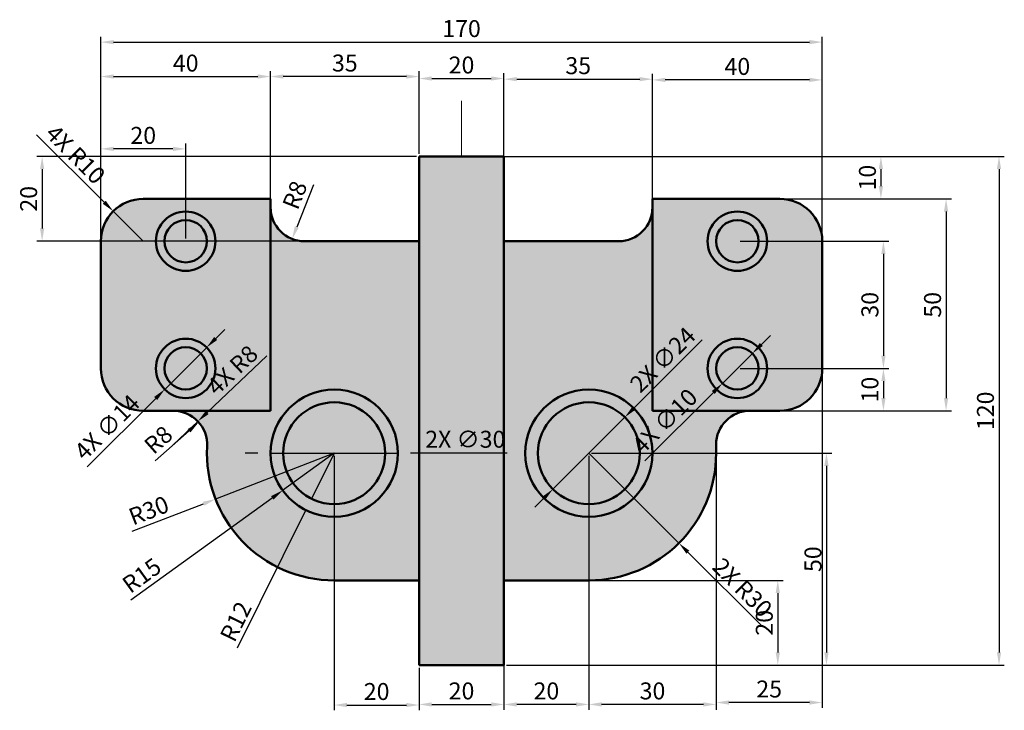
# Model space of a CAD drawing. Units: millimetres. Extents: x 624 to 856, y 718 to 881.
import ezdxf

# ---------------------------------------------------------------- set-up
doc = ezdxf.new("R2010")
doc.units = ezdxf.units.MM
doc.linetypes.add('CENTER', pattern=[50.8, 31.75, -6.35, 6.35, -6.35])
for name, color, linetype, lineweight in [('M-CNTR', 4, 'CENTER', 18), ('M-DIMS', 2, 'Continuous', 25), ('M-HATC', 8, 'Continuous', 18), ('M-OUTL', 7, 'Continuous', 50)]:
    doc.layers.add(name, color=color, linetype=linetype, lineweight=lineweight)
doc.styles.get("Standard").update_dxf_attribs({"font": 'arial.ttf'})
doc.dimstyles.new('ISO-25', dxfattribs={"dimtxt": 4, "dimasz": 3, "dimexe": 1.25, "dimexo": 0.625, "dimtad": 1, "dimdec": 1, "dimtxsty": 'Standard', "dimcen": 2.5, "dimadec": 0, "dimazin": 0, "dimtfac": 1, "dimtdec": 1, "dimtmove": 0, "dimatfit": 3, "dimfxl": 1, "dimarcsym": 0})

# ---------------------------------------------------------------- blocks, each defined once
blk = doc.blocks.new('*D1')
at = {"layer": 'Defpoints', "color": 0, "transparency": 16777216}
for p in [(698.17, 778.8), (718.17, 728.8), (718.17, 719.4)]:
    blk.add_point(p, dxfattribs=at)
at = {"layer": 'M-DIMS', "color": 0, "lineweight": -2, "transparency": 16777216}
for p, q in [((698.17, 778.17), (698.17, 718.15)), ((718.17, 728.17), (718.17, 718.15)), ((701.17, 719.4), (715.17, 719.4))]:
    blk.add_line(p, q, dxfattribs=at)
at = {"layer": 'M-DIMS', "color": 0, "transparency": 16777216}
for points in [[(701.17, 719.9), (701.17, 718.9), (698.17, 719.4)], [(715.17, 719.9), (715.17, 718.9), (718.17, 719.4)]]:
    blk.add_solid(points, dxfattribs=at)
at = {"layer": 'M-DIMS', "color": 0, "transparency": 16777216, "insert": (708.17, 722.07), "char_height": 4, "attachment_point": 5}
blk.add_mtext('20', dxfattribs=at)
blk = doc.blocks.new('*D2')
at = {"layer": 'Defpoints', "color": 0, "transparency": 16777216}
for p in [(738.17, 728.8), (718.17, 723.16), (738.17, 719.54)]:
    blk.add_point(p, dxfattribs=at)
at = {"layer": 'M-DIMS', "color": 0, "lineweight": -2, "transparency": 16777216}
for p, q in [((738.17, 728.17), (738.17, 718.29)), ((718.17, 722.54), (718.17, 718.29)), ((721.17, 719.54), (735.17, 719.54))]:
    blk.add_line(p, q, dxfattribs=at)
at = {"layer": 'M-DIMS', "color": 0, "transparency": 16777216}
for points in [[(721.17, 720.04), (721.17, 719.04), (718.17, 719.54)], [(735.17, 720.04), (735.17, 719.04), (738.17, 719.54)]]:
    blk.add_solid(points, dxfattribs=at)
at = {"layer": 'M-DIMS', "color": 0, "transparency": 16777216, "insert": (728.17, 722.21), "char_height": 4, "attachment_point": 5}
blk.add_mtext('20', dxfattribs=at)
blk = doc.blocks.new('*D3')
at = {"layer": 'Defpoints', "color": 0, "transparency": 16777216}
for p in [(758.17, 778.8), (738.17, 732.79), (738.17, 719.54)]:
    blk.add_point(p, dxfattribs=at)
at = {"layer": 'M-DIMS', "color": 0, "lineweight": -2, "transparency": 16777216}
for p, q in [((758.17, 778.17), (758.17, 718.29)), ((738.17, 732.16), (738.17, 718.29)), ((755.17, 719.54), (741.17, 719.54))]:
    blk.add_line(p, q, dxfattribs=at)
at = {"layer": 'M-DIMS', "color": 0, "transparency": 16777216}
for points in [[(741.17, 720.04), (741.17, 719.04), (738.17, 719.54)], [(755.17, 720.04), (755.17, 719.04), (758.17, 719.54)]]:
    blk.add_solid(points, dxfattribs=at)
at = {"layer": 'M-DIMS', "color": 0, "transparency": 16777216, "insert": (748.17, 722.21), "char_height": 4, "attachment_point": 5}
blk.add_mtext('20', dxfattribs=at)
blk = doc.blocks.new('*D4')
at = {"layer": 'Defpoints', "color": 0, "transparency": 16777216}
for p in [(788.17, 778.8), (758.17, 736.06), (758.17, 719.54)]:
    blk.add_point(p, dxfattribs=at)
at = {"layer": 'M-DIMS', "color": 0, "lineweight": -2, "transparency": 16777216}
for p, q in [((788.17, 778.17), (788.17, 718.29)), ((758.17, 735.44), (758.17, 718.29)), ((785.17, 719.54), (761.17, 719.54))]:
    blk.add_line(p, q, dxfattribs=at)
at = {"layer": 'M-DIMS', "color": 0, "transparency": 16777216}
for points in [[(761.17, 720.04), (761.17, 719.04), (758.17, 719.54)], [(785.17, 720.04), (785.17, 719.04), (788.17, 719.54)]]:
    blk.add_solid(points, dxfattribs=at)
at = {"layer": 'M-DIMS', "color": 0, "transparency": 16777216, "insert": (773.17, 722.21), "char_height": 4, "attachment_point": 5}
blk.add_mtext('30', dxfattribs=at)
blk = doc.blocks.new('*D5')
at = {"layer": 'Defpoints', "color": 0, "transparency": 16777216}
for p in [(758.17, 778.8), (738.17, 728.8), (814.17, 728.8)]:
    blk.add_point(p, dxfattribs=at)
at = {"layer": 'M-DIMS', "color": 0, "lineweight": -2, "transparency": 16777216}
for p, q in [((758.8, 778.8), (815.42, 778.8)), ((814.17, 775.8), (814.17, 731.8)), ((738.8, 728.8), (815.42, 728.8))]:
    blk.add_line(p, q, dxfattribs=at)
at = {"layer": 'M-DIMS', "color": 0, "transparency": 16777216}
for points in [[(813.67, 775.8), (814.67, 775.8), (814.17, 778.8)], [(813.67, 731.8), (814.67, 731.8), (814.17, 728.8)]]:
    blk.add_solid(points, dxfattribs=at)
at = {"layer": 'M-DIMS', "color": 0, "transparency": 16777216, "insert": (811.51, 753.8), "char_height": 4, "attachment_point": 5, "rotation": 90}
blk.add_mtext('50', dxfattribs=at)
blk = doc.blocks.new('*D6')
at = {"layer": 'Defpoints', "color": 0, "transparency": 16777216}
for p in [(749.94, 748.8), (749.94, 728.8), (802.7, 728.8)]:
    blk.add_point(p, dxfattribs=at)
at = {"layer": 'M-DIMS', "color": 0, "lineweight": -2, "transparency": 16777216}
for p, q in [((750.56, 748.8), (803.95, 748.8)), ((802.7, 745.8), (802.7, 731.8)), ((750.56, 728.8), (803.95, 728.8))]:
    blk.add_line(p, q, dxfattribs=at)
at = {"layer": 'M-DIMS', "color": 0, "transparency": 16777216}
for points in [[(802.2, 745.8), (803.2, 745.8), (802.7, 748.8)], [(802.2, 731.8), (803.2, 731.8), (802.7, 728.8)]]:
    blk.add_solid(points, dxfattribs=at)
at = {"layer": 'M-DIMS', "color": 0, "transparency": 16777216, "insert": (800.04, 738.8), "char_height": 4, "attachment_point": 5, "rotation": 90}
blk.add_mtext('20', dxfattribs=at)
blk = doc.blocks.new('*D7')
at = {"layer": 'Defpoints', "color": 0, "transparency": 16777216}
for p in [(793.17, 798.8), (800.11, 788.8), (827.59, 788.8)]:
    blk.add_point(p, dxfattribs=at)
at = {"layer": 'M-DIMS', "color": 0, "lineweight": -2, "transparency": 16777216}
for p, q in [((793.8, 798.8), (828.84, 798.8)), ((827.59, 795.8), (827.59, 791.8)), ((800.74, 788.8), (828.84, 788.8))]:
    blk.add_line(p, q, dxfattribs=at)
at = {"layer": 'M-DIMS', "color": 0, "transparency": 16777216}
for points in [[(827.09, 795.8), (828.09, 795.8), (827.59, 798.8)], [(827.09, 791.8), (828.09, 791.8), (827.59, 788.8)]]:
    blk.add_solid(points, dxfattribs=at)
at = {"layer": 'M-DIMS', "color": 0, "transparency": 16777216, "insert": (824.92, 793.8), "char_height": 4, "attachment_point": 5, "rotation": 90}
blk.add_mtext('10', dxfattribs=at)
blk = doc.blocks.new('*D8')
at = {"layer": 'Defpoints', "color": 0, "transparency": 16777216}
for p in [(793.17, 828.8), (793.17, 798.8), (827.59, 798.8)]:
    blk.add_point(p, dxfattribs=at)
at = {"layer": 'M-DIMS', "color": 0, "lineweight": -2, "transparency": 16777216}
for p, q in [((793.8, 828.8), (828.84, 828.8)), ((827.59, 825.8), (827.59, 801.8)), ((793.8, 798.8), (828.84, 798.8))]:
    blk.add_line(p, q, dxfattribs=at)
at = {"layer": 'M-DIMS', "color": 0, "transparency": 16777216}
for points in [[(827.09, 825.8), (828.09, 825.8), (827.59, 828.8)], [(827.09, 801.8), (828.09, 801.8), (827.59, 798.8)]]:
    blk.add_solid(points, dxfattribs=at)
at = {"layer": 'M-DIMS', "color": 0, "transparency": 16777216, "insert": (824.92, 813.8), "char_height": 4, "attachment_point": 5, "rotation": 90}
blk.add_mtext('30', dxfattribs=at)
blk = doc.blocks.new('*D9')
at = {"layer": 'Defpoints', "color": 0, "transparency": 16777216}
for p in [(794.11, 838.8), (798.04, 788.8), (842.36, 788.8)]:
    blk.add_point(p, dxfattribs=at)
at = {"layer": 'M-DIMS', "color": 0, "lineweight": -2, "transparency": 16777216}
for p, q in [((794.74, 838.8), (843.61, 838.8)), ((842.36, 835.8), (842.36, 791.8)), ((798.66, 788.8), (843.61, 788.8))]:
    blk.add_line(p, q, dxfattribs=at)
at = {"layer": 'M-DIMS', "color": 0, "transparency": 16777216}
for points in [[(841.86, 835.8), (842.86, 835.8), (842.36, 838.8)], [(841.86, 791.8), (842.86, 791.8), (842.36, 788.8)]]:
    blk.add_solid(points, dxfattribs=at)
at = {"layer": 'M-DIMS', "color": 0, "transparency": 16777216, "insert": (839.69, 813.8), "char_height": 4, "attachment_point": 5, "rotation": 90}
blk.add_mtext('50', dxfattribs=at)
blk = doc.blocks.new('*D10')
at = {"layer": 'Defpoints', "color": 0, "transparency": 16777216}
for p in [(728.17, 848.8), (795.5, 728.8), (854.83, 728.8)]:
    blk.add_point(p, dxfattribs=at)
at = {"layer": 'M-DIMS', "color": 0, "lineweight": -2, "transparency": 16777216}
for p, q in [((728.8, 848.8), (856.08, 848.8)), ((854.83, 845.8), (854.83, 731.8)), ((796.12, 728.8), (856.08, 728.8))]:
    blk.add_line(p, q, dxfattribs=at)
at = {"layer": 'M-DIMS', "color": 0, "transparency": 16777216}
for points in [[(854.33, 845.8), (855.33, 845.8), (854.83, 848.8)], [(854.33, 731.8), (855.33, 731.8), (854.83, 728.8)]]:
    blk.add_solid(points, dxfattribs=at)
at = {"layer": 'M-DIMS', "color": 0, "transparency": 16777216, "insert": (852.16, 788.8), "char_height": 4, "attachment_point": 5, "rotation": 90}
blk.add_mtext('120', dxfattribs=at)
blk = doc.blocks.new('*D11')
at = {"layer": 'Defpoints', "color": 0, "transparency": 16777216}
for p in [(683.17, 867.64), (643.17, 820.21), (683.17, 818.82)]:
    blk.add_point(p, dxfattribs=at)
at = {"layer": 'M-DIMS', "color": 0, "lineweight": -2, "transparency": 16777216}
for p, q in [((643.17, 820.83), (643.17, 868.89)), ((683.17, 819.44), (683.17, 868.89)), ((646.17, 867.64), (680.17, 867.64))]:
    blk.add_line(p, q, dxfattribs=at)
at = {"layer": 'M-DIMS', "color": 0, "transparency": 16777216}
for points in [[(646.17, 868.14), (646.17, 867.14), (643.17, 867.64)], [(680.17, 868.14), (680.17, 867.14), (683.17, 867.64)]]:
    blk.add_solid(points, dxfattribs=at)
at = {"layer": 'M-DIMS', "color": 0, "transparency": 16777216, "insert": (663.17, 870.3), "char_height": 4, "attachment_point": 5}
blk.add_mtext('40', dxfattribs=at)
blk = doc.blocks.new('*D12')
at = {"layer": 'Defpoints', "color": 0, "transparency": 16777216}
for p in [(683.17, 867.64), (683.17, 848.8), (718.17, 848.8)]:
    blk.add_point(p, dxfattribs=at)
at = {"layer": 'M-DIMS', "color": 0, "lineweight": -2, "transparency": 16777216}
for p, q in [((683.17, 849.42), (683.17, 868.89)), ((718.17, 849.42), (718.17, 868.89)), ((715.17, 867.64), (686.17, 867.64))]:
    blk.add_line(p, q, dxfattribs=at)
at = {"layer": 'M-DIMS', "color": 0, "transparency": 16777216}
for points in [[(686.17, 868.14), (686.17, 867.14), (683.17, 867.64)], [(715.17, 868.14), (715.17, 867.14), (718.17, 867.64)]]:
    blk.add_solid(points, dxfattribs=at)
at = {"layer": 'M-DIMS', "color": 0, "transparency": 16777216, "insert": (700.67, 870.31), "char_height": 4, "attachment_point": 5}
blk.add_mtext('35', dxfattribs=at)
blk = doc.blocks.new('*D13')
at = {"layer": 'Defpoints', "color": 0, "transparency": 16777216}
for p in [(738.17, 867.17), (718.17, 848.8), (738.17, 848.8)]:
    blk.add_point(p, dxfattribs=at)
at = {"layer": 'M-DIMS', "color": 0, "lineweight": -2, "transparency": 16777216}
for p, q in [((718.17, 849.42), (718.17, 868.42)), ((738.17, 849.42), (738.17, 868.42)), ((721.17, 867.17), (735.17, 867.17))]:
    blk.add_line(p, q, dxfattribs=at)
at = {"layer": 'M-DIMS', "color": 0, "transparency": 16777216}
for points in [[(721.17, 867.67), (721.17, 866.67), (718.17, 867.17)], [(735.17, 867.67), (735.17, 866.67), (738.17, 867.17)]]:
    blk.add_solid(points, dxfattribs=at)
at = {"layer": 'M-DIMS', "color": 0, "transparency": 16777216, "insert": (728.17, 869.84), "char_height": 4, "attachment_point": 5}
blk.add_mtext('20', dxfattribs=at)
blk = doc.blocks.new('*D14')
at = {"layer": 'Defpoints', "color": 0, "transparency": 16777216}
for p in [(773.17, 867.02), (738.17, 839.17), (773.17, 838.8)]:
    blk.add_point(p, dxfattribs=at)
at = {"layer": 'M-DIMS', "color": 0, "lineweight": -2, "transparency": 16777216}
for p, q in [((738.17, 839.79), (738.17, 868.27)), ((773.17, 839.42), (773.17, 868.27)), ((741.17, 867.02), (770.17, 867.02))]:
    blk.add_line(p, q, dxfattribs=at)
at = {"layer": 'M-DIMS', "color": 0, "transparency": 16777216}
for points in [[(741.17, 867.52), (741.17, 866.52), (738.17, 867.02)], [(770.17, 867.52), (770.17, 866.52), (773.17, 867.02)]]:
    blk.add_solid(points, dxfattribs=at)
at = {"layer": 'M-DIMS', "color": 0, "transparency": 16777216, "insert": (755.67, 869.69), "char_height": 4, "attachment_point": 5}
blk.add_mtext('35', dxfattribs=at)
blk = doc.blocks.new('*D15')
at = {"layer": 'Defpoints', "color": 0, "transparency": 16777216}
for p in [(773.17, 866.84), (773.17, 818.33), (813.17, 818.33)]:
    blk.add_point(p, dxfattribs=at)
at = {"layer": 'M-DIMS', "color": 0, "lineweight": -2, "transparency": 16777216}
for p, q in [((773.17, 818.95), (773.17, 868.09)), ((813.17, 818.95), (813.17, 868.09)), ((810.17, 866.84), (776.17, 866.84))]:
    blk.add_line(p, q, dxfattribs=at)
at = {"layer": 'M-DIMS', "color": 0, "transparency": 16777216}
for points in [[(776.17, 867.34), (776.17, 866.34), (773.17, 866.84)], [(810.17, 867.34), (810.17, 866.34), (813.17, 866.84)]]:
    blk.add_solid(points, dxfattribs=at)
at = {"layer": 'M-DIMS', "color": 0, "transparency": 16777216, "insert": (793.17, 869.51), "char_height": 4, "attachment_point": 5}
blk.add_mtext('40', dxfattribs=at)
blk = doc.blocks.new('*D16')
at = {"layer": 'Defpoints', "color": 0, "transparency": 16777216}
for p in [(643.17, 850.58), (663.17, 828.8), (643.17, 816.04)]:
    blk.add_point(p, dxfattribs=at)
at = {"layer": 'M-DIMS', "color": 0, "lineweight": -2, "transparency": 16777216}
for p, q in [((643.17, 816.67), (643.17, 851.83)), ((663.17, 829.42), (663.17, 851.83)), ((660.17, 850.58), (646.17, 850.58))]:
    blk.add_line(p, q, dxfattribs=at)
at = {"layer": 'M-DIMS', "color": 0, "transparency": 16777216}
for points in [[(646.17, 851.08), (646.17, 850.08), (643.17, 850.58)], [(660.17, 851.08), (660.17, 850.08), (663.17, 850.58)]]:
    blk.add_solid(points, dxfattribs=at)
at = {"layer": 'M-DIMS', "color": 0, "transparency": 16777216, "insert": (653.17, 853.24), "char_height": 4, "attachment_point": 5}
blk.add_mtext('20', dxfattribs=at)
blk = doc.blocks.new('*D17')
at = {"layer": 'Defpoints', "color": 0, "transparency": 16777216}
for p in [(691.17, 836.8), (688.24, 829.35)]:
    blk.add_point(p, dxfattribs=at)
at = {"layer": 'M-DIMS', "color": 0, "lineweight": -2, "transparency": 16777216}
blk.add_line((693.27, 842.11), (689.34, 832.14), dxfattribs=at)
at = {"layer": 'M-DIMS', "color": 0, "transparency": 16777216}
blk.add_solid([(688.88, 832.33), (689.81, 831.96), (688.24, 829.35)], dxfattribs=at)
at = {"layer": 'M-DIMS', "color": 0, "transparency": 16777216, "insert": (689.37, 839.5), "char_height": 4, "attachment_point": 5, "rotation": 68.4911}
blk.add_mtext('R8', dxfattribs=at)
blk = doc.blocks.new('*D18')
at = {"layer": 'Defpoints', "color": 0, "transparency": 16777216}
for p in [(698.17, 778.8), (686.01, 770.02)]:
    blk.add_point(p, dxfattribs=at)
at = {"layer": 'M-DIMS', "color": 0, "lineweight": -2, "transparency": 16777216}
for p, q in [((698.17, 778.8), (686.01, 770.02)), ((650.28, 744.22), (683.58, 768.26))]:
    blk.add_line(p, q, dxfattribs=at)
at = {"layer": 'M-DIMS', "color": 0, "transparency": 16777216}
blk.add_solid([(683.29, 768.67), (683.87, 767.85), (686.01, 770.02)], dxfattribs=at)
at = {"layer": 'M-DIMS', "color": 0, "transparency": 16777216, "insert": (653.11, 749.55), "char_height": 4, "attachment_point": 5, "rotation": 35.8278}
blk.add_mtext('R15', dxfattribs=at)
blk = doc.blocks.new('*D19')
at = {"layer": 'Defpoints', "color": 0, "transparency": 16777216}
for p in [(698.17, 778.8), (692.85, 768.04)]:
    blk.add_point(p, dxfattribs=at)
at = {"layer": 'M-DIMS', "color": 0, "lineweight": -2, "transparency": 16777216}
for p, q in [((698.17, 778.8), (692.85, 768.04)), ((675.41, 732.87), (691.51, 765.36))]:
    blk.add_line(p, q, dxfattribs=at)
at = {"layer": 'M-DIMS', "color": 0, "transparency": 16777216}
blk.add_solid([(691.06, 765.58), (691.96, 765.13), (692.85, 768.04)], dxfattribs=at)
at = {"layer": 'M-DIMS', "color": 0, "transparency": 16777216, "insert": (675.44, 738.87), "char_height": 4, "attachment_point": 5, "rotation": 63.6308}
blk.add_mtext('R12', dxfattribs=at)
blk = doc.blocks.new('*D20')
at = {"layer": 'Defpoints', "color": 0, "transparency": 16777216}
for p in [(698.17, 778.8), (670.2, 767.97)]:
    blk.add_point(p, dxfattribs=at)
at = {"layer": 'M-DIMS', "color": 0, "lineweight": -2, "transparency": 16777216}
for p, q in [((698.17, 778.8), (670.2, 767.97)), ((650.58, 760.38), (667.4, 766.89))]:
    blk.add_line(p, q, dxfattribs=at)
at = {"layer": 'M-DIMS', "color": 0, "transparency": 16777216}
blk.add_solid([(667.22, 767.35), (667.58, 766.42), (670.2, 767.97)], dxfattribs=at)
at = {"layer": 'M-DIMS', "color": 0, "transparency": 16777216, "insert": (654.65, 764.81), "char_height": 4, "attachment_point": 5, "rotation": 21.1564}
blk.add_mtext('R30', dxfattribs=at)
blk = doc.blocks.new('*D21')
at = {"layer": 'Defpoints', "color": 0, "transparency": 16777216}
for p in [(666.22, 786.09), (660.23, 780.8)]:
    blk.add_point(p, dxfattribs=at)
at = {"layer": 'M-DIMS', "color": 0, "lineweight": -2, "transparency": 16777216}
blk.add_line((655.95, 777.02), (663.98, 784.11), dxfattribs=at)
at = {"layer": 'M-DIMS', "color": 0, "transparency": 16777216}
blk.add_solid([(663.64, 784.48), (664.31, 783.73), (666.22, 786.09)], dxfattribs=at)
at = {"layer": 'M-DIMS', "color": 0, "transparency": 16777216, "insert": (657.07, 781.57), "char_height": 4, "attachment_point": 5, "rotation": 41.4423}
blk.add_mtext('R8', dxfattribs=at)
blk = doc.blocks.new('*D22')
at = {"layer": 'Defpoints', "color": 0, "transparency": 16777216}
for p in [(813.17, 813.8), (788.17, 723.81), (788.17, 719.99)]:
    blk.add_point(p, dxfattribs=at)
at = {"layer": 'M-DIMS', "color": 0, "lineweight": -2, "transparency": 16777216}
for p, q in [((813.17, 813.17), (813.17, 718.74)), ((788.17, 723.19), (788.17, 718.74)), ((810.17, 719.99), (791.17, 719.99))]:
    blk.add_line(p, q, dxfattribs=at)
at = {"layer": 'M-DIMS', "color": 0, "transparency": 16777216}
for points in [[(791.17, 720.49), (791.17, 719.49), (788.17, 719.99)], [(810.17, 720.49), (810.17, 719.49), (813.17, 719.99)]]:
    blk.add_solid(points, dxfattribs=at)
at = {"layer": 'M-DIMS', "color": 0, "transparency": 16777216, "insert": (800.67, 722.66), "char_height": 4, "attachment_point": 5}
blk.add_mtext('25', dxfattribs=at)
blk = doc.blocks.new('CLEVIS-LUG-40X50-2HOLE')
for p, q in [((10, 50), (40, 50)), ((40, 0), (40, 50)), ((0, 40), (0, 10)), ((10, 0), (40, 0))]:
    blk.add_line(p, q)
for centre, radius in [((20, 40), 7), ((20, 40), 5), ((20, 10), 7), ((20, 10), 5)]:
    blk.add_circle(centre, radius)
for centre, start, end in [((10, 40), 90, 180), ((10, 10), 180, 270)]:
    blk.add_arc(centre, 10, start, end)
blk = doc.blocks.new('PLATE-BORE-D24-D30')
for radius in [15, 12]:
    blk.add_circle((15, 15), radius)
blk = doc.blocks.new('*D25')
at = {"layer": 'Defpoints', "color": 0, "transparency": 16777216}
for p in [(813.17, 875.76), (643.17, 828.8), (813.17, 828.8)]:
    blk.add_point(p, dxfattribs=at)
at = {"layer": 'M-DIMS', "color": 0, "lineweight": -2, "transparency": 16777216}
for p, q in [((643.17, 829.42), (643.17, 877.01)), ((646.17, 875.76), (810.17, 875.76)), ((813.17, 829.42), (813.17, 877.01))]:
    blk.add_line(p, q, dxfattribs=at)
at = {"layer": 'M-DIMS', "color": 0, "transparency": 16777216}
for points in [[(646.17, 876.26), (646.17, 875.26), (643.17, 875.76)], [(810.17, 876.26), (810.17, 875.26), (813.17, 875.76)]]:
    blk.add_solid(points, dxfattribs=at)
at = {"layer": 'M-DIMS', "color": 0, "transparency": 16777216, "insert": (728.17, 878.43), "char_height": 4, "attachment_point": 5}
blk.add_mtext('170', dxfattribs=at)
blk = doc.blocks.new('*D26')
at = {"layer": 'Defpoints', "color": 0, "transparency": 16777216}
for p in [(738.17, 848.8), (803.17, 838.8), (827, 838.8)]:
    blk.add_point(p, dxfattribs=at)
at = {"layer": 'M-DIMS', "color": 0, "lineweight": -2, "transparency": 16777216}
for p, q in [((738.8, 848.8), (828.25, 848.8)), ((827, 845.8), (827, 841.8)), ((803.8, 838.8), (828.25, 838.8))]:
    blk.add_line(p, q, dxfattribs=at)
at = {"layer": 'M-DIMS', "color": 0, "transparency": 16777216}
for points in [[(826.5, 845.8), (827.5, 845.8), (827, 848.8)], [(826.5, 841.8), (827.5, 841.8), (827, 838.8)]]:
    blk.add_solid(points, dxfattribs=at)
at = {"layer": 'M-DIMS', "color": 0, "transparency": 16777216, "insert": (824.34, 843.8), "char_height": 4, "attachment_point": 5, "rotation": 90}
blk.add_mtext('10', dxfattribs=at)
blk = doc.blocks.new('*D27')
at = {"layer": 'Defpoints', "color": 0, "transparency": 16777216}
for p in [(718.17, 848.8), (629.34, 828.8), (718.17, 828.8)]:
    blk.add_point(p, dxfattribs=at)
at = {"layer": 'M-DIMS', "color": 0, "lineweight": -2, "transparency": 16777216}
for p, q in [((717.55, 848.8), (628.09, 848.8)), ((629.34, 845.8), (629.34, 831.8)), ((717.55, 828.8), (628.09, 828.8))]:
    blk.add_line(p, q, dxfattribs=at)
at = {"layer": 'M-DIMS', "color": 0, "transparency": 16777216}
for points in [[(628.84, 845.8), (629.84, 845.8), (629.34, 848.8)], [(628.84, 831.8), (629.84, 831.8), (629.34, 828.8)]]:
    blk.add_solid(points, dxfattribs=at)
at = {"layer": 'M-DIMS', "color": 0, "transparency": 16777216, "insert": (626.68, 838.8), "char_height": 4, "attachment_point": 5, "rotation": 90}
blk.add_mtext('20', dxfattribs=at)
blk = doc.blocks.new('*D28')
at = {"layer": 'Defpoints', "color": 0, "transparency": 16777216}
for p in [(758.17, 778.8), (779.39, 757.58)]:
    blk.add_point(p, dxfattribs=at)
at = {"layer": 'M-DIMS', "color": 0, "lineweight": -2, "transparency": 16777216}
for p, q in [((758.17, 778.8), (779.39, 757.58)), ((799, 737.98), (781.51, 755.46))]:
    blk.add_line(p, q, dxfattribs=at)
at = {"layer": 'M-DIMS', "color": 0, "transparency": 16777216}
blk.add_solid([(781.86, 755.82), (781.16, 755.11), (779.39, 757.58)], dxfattribs=at)
at = {"layer": 'M-DIMS', "color": 0, "transparency": 16777216, "insert": (794, 746.74), "char_height": 4, "attachment_point": 5, "rotation": 314.9999}
blk.add_mtext('2X R30', dxfattribs=at)
blk = doc.blocks.new('*D29')
at = {"layer": 'Defpoints', "color": 0, "transparency": 16777216}
for p in [(646.1, 835.87), (653.17, 828.8)]:
    blk.add_point(p, dxfattribs=at)
at = {"layer": 'M-DIMS', "color": 0, "lineweight": -2, "transparency": 16777216}
for p, q in [((628.04, 853.93), (643.98, 837.99)), ((653.17, 828.8), (646.1, 835.87))]:
    blk.add_line(p, q, dxfattribs=at)
at = {"layer": 'M-DIMS', "color": 0, "transparency": 16777216}
blk.add_solid([(644.34, 838.34), (643.63, 837.63), (646.1, 835.87)], dxfattribs=at)
at = {"layer": 'M-DIMS', "color": 0, "transparency": 16777216, "insert": (636.84, 848.91), "char_height": 4, "attachment_point": 5, "rotation": 315.0003}
blk.add_mtext('4X R10', dxfattribs=at)
blk = doc.blocks.new('*D30')
at = {"layer": 'Defpoints', "color": 0, "transparency": 16777216}
for p in [(666.03, 786.3), (660.23, 780.8)]:
    blk.add_point(p, dxfattribs=at)
at = {"layer": 'M-DIMS', "color": 0, "lineweight": -2, "transparency": 16777216}
for p, q in [((682.33, 801.76), (668.21, 788.37)), ((660.23, 780.8), (666.03, 786.3))]:
    blk.add_line(p, q, dxfattribs=at)
at = {"layer": 'M-DIMS', "color": 0, "transparency": 16777216}
blk.add_solid([(667.86, 788.73), (668.55, 788), (666.03, 786.3)], dxfattribs=at)
at = {"layer": 'M-DIMS', "color": 0, "transparency": 16777216, "insert": (674.52, 798.03), "char_height": 4, "attachment_point": 5, "rotation": 43.4923}
blk.add_mtext('4X R8', dxfattribs=at)
blk = doc.blocks.new('*D31')
at = {"layer": 'Defpoints', "color": 0, "transparency": 16777216}
for p in [(683.17, 778.8), (713.17, 778.8)]:
    blk.add_point(p, dxfattribs=at)
at = {"layer": 'M-DIMS', "color": 0, "lineweight": -2, "transparency": 16777216}
for p, q in [((680.17, 778.8), (677.17, 778.8)), ((683.17, 778.8), (713.17, 778.8)), ((738.94, 778.8), (716.17, 778.8))]:
    blk.add_line(p, q, dxfattribs=at)
at = {"layer": 'M-DIMS', "color": 0, "transparency": 16777216}
for points in [[(680.17, 779.3), (680.17, 778.3), (683.17, 778.8)], [(716.17, 779.3), (716.17, 778.3), (713.17, 778.8)]]:
    blk.add_solid(points, dxfattribs=at)
at = {"layer": 'M-DIMS', "color": 0, "transparency": 16777216, "insert": (729.06, 781.57), "char_height": 4, "attachment_point": 5, "rotation": 359.9992}
blk.add_mtext('2X ∅30', dxfattribs=at)
blk = doc.blocks.new('*D32')
at = {"layer": 'Defpoints', "color": 0, "transparency": 16777216}
for p in [(766.66, 787.28), (749.69, 770.31)]:
    blk.add_point(p, dxfattribs=at)
at = {"layer": 'M-DIMS', "color": 0, "lineweight": -2, "transparency": 16777216}
for p, q in [((784.88, 805.5), (768.78, 789.4)), ((749.69, 770.31), (766.66, 787.28)), ((747.57, 768.19), (745.45, 766.07))]:
    blk.add_line(p, q, dxfattribs=at)
at = {"layer": 'M-DIMS', "color": 0, "transparency": 16777216}
for points in [[(768.43, 789.76), (769.14, 789.05), (766.66, 787.28)], [(747.21, 768.54), (747.92, 767.84), (749.69, 770.31)]]:
    blk.add_solid(points, dxfattribs=at)
at = {"layer": 'M-DIMS', "color": 0, "transparency": 16777216, "insert": (775.93, 800.48), "char_height": 4, "attachment_point": 5, "rotation": 44.9955}
blk.add_mtext('2X ∅24', dxfattribs=at)
blk = doc.blocks.new('*D33')
at = {"layer": 'Defpoints', "color": 0, "transparency": 16777216}
for p in [(668.12, 803.75), (658.23, 793.85)]:
    blk.add_point(p, dxfattribs=at)
at = {"layer": 'M-DIMS', "color": 0, "lineweight": -2, "transparency": 16777216}
for p, q in [((670.25, 805.87), (672.37, 807.99)), ((668.12, 803.75), (658.23, 793.85)), ((639.94, 775.56), (656.1, 791.72))]:
    blk.add_line(p, q, dxfattribs=at)
at = {"layer": 'M-DIMS', "color": 0, "transparency": 16777216}
for points in [[(669.89, 806.22), (670.6, 805.51), (668.12, 803.75)], [(655.75, 792.08), (656.46, 791.37), (658.23, 793.85)]]:
    blk.add_solid(points, dxfattribs=at)
at = {"layer": 'M-DIMS', "color": 0, "transparency": 16777216, "insert": (645, 784.55), "char_height": 4, "attachment_point": 5, "rotation": 45.0019}
blk.add_mtext('4X ∅14', dxfattribs=at)
blk = doc.blocks.new('*D34')
at = {"layer": 'Defpoints', "color": 0, "transparency": 16777216}
for p in [(796.71, 802.33), (789.64, 795.26)]:
    blk.add_point(p, dxfattribs=at)
at = {"layer": 'M-DIMS', "color": 0, "lineweight": -2, "transparency": 16777216}
for p, q in [((798.83, 804.45), (800.95, 806.57)), ((796.71, 802.33), (789.64, 795.26)), ((771.35, 776.97), (787.52, 793.14))]:
    blk.add_line(p, q, dxfattribs=at)
at = {"layer": 'M-DIMS', "color": 0, "transparency": 16777216}
for points in [[(798.48, 804.81), (799.19, 804.1), (796.71, 802.33)], [(787.16, 793.49), (787.87, 792.79), (789.64, 795.26)]]:
    blk.add_solid(points, dxfattribs=at)
at = {"layer": 'M-DIMS', "color": 0, "transparency": 16777216, "insert": (776.41, 785.96), "char_height": 4, "attachment_point": 5, "rotation": 45.0027}
blk.add_mtext('4X ∅10', dxfattribs=at)

msp = doc.modelspace()

# ---------------------------------------------------------------- hatches: boundary and pattern name
at = {"layer": 'M-HATC'}
h = msp.add_hatch(color=256, dxfattribs=at)
h.set_gradient(color1=(192, 192, 192), color2=(192, 192, 192), tint=1, name='CYLINDER')
h.paths.add_polyline_path([(718.17, 728.8), (738.17, 728.8), (738.17, 848.8), (718.17, 848.8)])
h.paths.add_polyline_path([(743.17, 778.8, 1), (773.17, 778.8, 1)])
h.paths.add_polyline_path([(770.17, 778.8, -1), (746.17, 778.8, -1)], flags=16)
h.paths.add_polyline_path([(683.17, 778.8, 1), (713.17, 778.8, 1)])
h.paths.add_polyline_path([(710.17, 778.8, -1), (686.17, 778.8, -1)], flags=16)
h = msp.add_hatch(color=256, dxfattribs=at)
h.set_gradient(color1=(0, 255, 0), color2=(255, 255, 0), tint=1, name='CYLINDER')
h.paths.add_polyline_path([(683.17, 838.8), (653.17, 838.8, 0.414214), (643.17, 828.8), (643.17, 798.8, 0.414214), (653.17, 788.8), (683.17, 788.8)])
h.paths.add_polyline_path([(670.17, 798.8, -1), (656.17, 798.8, -1)], flags=16)
h.paths.add_polyline_path([(668.17, 798.8, -1), (658.17, 798.8, -1)], flags=0)
h.paths.add_polyline_path([(656.17, 828.8, -1), (670.17, 828.8, -1)], flags=16)
h.paths.add_polyline_path([(658.17, 828.8, -1), (668.17, 828.8, -1)], flags=0)
h.paths.add_polyline_path([(813.17, 828.8, 0.414214), (803.17, 838.8), (773.17, 838.8), (773.17, 788.8), (803.17, 788.8, 0.414214), (813.17, 798.8)])
h.paths.add_polyline_path([(800.17, 798.8, -1), (786.17, 798.8, -1)], flags=16)
h.paths.add_polyline_path([(798.17, 798.8, -1), (788.17, 798.8, -1)], flags=0)
h.paths.add_polyline_path([(786.17, 828.8, -1), (800.17, 828.8, -1)], flags=16)
h.paths.add_polyline_path([(788.17, 828.8, -1), (798.17, 828.8, -1)], flags=0)
h = msp.add_hatch(color=256, dxfattribs=at)
h.set_gradient(color1=(237, 31, 36), color2=(241, 235, 31), tint=1, name='CYLINDER')
h.paths.add_polyline_path([(656.17, 828.8, 1), (670.17, 828.8, 1)])
h.paths.add_polyline_path([(668.17, 828.8, -1), (658.17, 828.8, -1)], flags=16)
h.paths.add_polyline_path([(670.17, 798.8, 1), (656.17, 798.8, 1)])
h.paths.add_polyline_path([(658.17, 798.8, -1), (668.17, 798.8, -1)], flags=16)
h.paths.add_polyline_path([(786.17, 798.8, 1), (800.17, 798.8, 1)])
h.paths.add_polyline_path([(798.17, 798.8, -1), (788.17, 798.8, -1)], flags=16)
h = msp.add_hatch(color=256, dxfattribs=at)
h.set_gradient(color1=(237, 31, 36), color2=(241, 235, 31), tint=1, name='CYLINDER')
h.paths.add_polyline_path([(668.17, 828.8, 1), (658.17, 828.8, 1)])
h.paths.add_polyline_path([(800.17, 828.8, 1), (786.17, 828.8, 1)])
h.paths.add_polyline_path([(788.17, 828.8, -1), (798.17, 828.8, -1)], flags=0)
h.paths.add_polyline_path([(788.17, 828.8, 1), (798.17, 828.8, 1)], flags=16)
h.paths.add_polyline_path([(668.17, 798.8, 1), (658.17, 798.8, 1)])
h.paths.add_polyline_path([(798.17, 798.8, 1), (788.17, 798.8, 1)])
h.paths.add_polyline_path([(718.17, 828.8), (691.17, 828.8, -0.414214), (683.17, 836.8), (683.17, 788.8), (660.23, 788.8, -0.429722), (668.22, 780.38, 0.429722), (698.17, 748.8), (718.17, 748.8)])
h.paths.add_polyline_path([(713.17, 778.8, -1), (683.17, 778.8, -1)], flags=16)
h.paths.add_polyline_path([(710.17, 778.8, -1), (686.17, 778.8, -1)], flags=0)
h.paths.add_polyline_path([(773.17, 836.8, -0.414214), (765.17, 828.8), (738.17, 828.8), (738.17, 748.8), (758.17, 748.8, 0.414214), (788.17, 778.8), (788.17, 780.8, -0.414214), (796.17, 788.8), (773.17, 788.8)])
h.paths.add_polyline_path([(773.17, 778.8, -1), (743.17, 778.8, -1)], flags=16)
h.paths.add_polyline_path([(770.17, 778.8, -1), (746.17, 778.8, -1)], flags=0)

# ---------------------------------------------------------------- linework, layer by layer
at = {"layer": 'M-CNTR'}
msp.add_line((728.17, 848.8), (728.17, 861.93), dxfattribs=at)
at = {"layer": 'M-OUTL'}
for p, q in [((718.17, 848.8), (718.17, 728.8)), ((718.17, 848.8), (738.17, 848.8)), ((738.17, 848.8), (738.17, 728.8)), ((683.17, 838.8), (683.17, 836.8)), ((773.17, 838.8), (773.17, 836.8)), ((691.17, 828.8), (718.17, 828.8)), ((738.17, 828.8), (765.17, 828.8)), ((788.17, 780.8), (788.17, 778.8)), ((718.17, 748.8), (698.17, 748.8)), ((738.17, 748.8), (758.17, 748.8)), ((718.17, 728.8), (738.17, 728.8))]:
    msp.add_line(p, q, dxfattribs=at)
for centre, radius, start, end in [((691.17, 836.8), 8, 180, 270), ((765.17, 836.8), 8, 270, 0), ((660.23, 780.8), 8, 356.983, 90), ((796.17, 780.8), 8, 90, 180), ((698.17, 778.8), 30, 176.983, 270), ((758.17, 778.8), 30, 270, 0)]:
    msp.add_arc(centre, radius, start, end, dxfattribs=at)

# ---------------------------------------------------------------- block references
for name, p in [('CLEVIS-LUG-40X50-2HOLE', (643.17, 788.8)), ('PLATE-BORE-D24-D30', (683.17, 763.8)), ('PLATE-BORE-D24-D30', (743.17, 763.8))]:
    msp.add_blockref(name, p, dxfattribs=at)
at = {"layer": 'M-OUTL', "rotation": 180}
msp.add_blockref('CLEVIS-LUG-40X50-2HOLE', (813.17, 838.8), dxfattribs=at)

# ---------------------------------------------------------------- dimensions: what is measured, and where the dimension line sits
at = {"layer": 'M-DIMS'}
for base, p1, p2, override, picture, middle in [((813.17, 875.76), (643.17, 828.8), (813.17, 828.8), {"dimdec": 0, "dimlfac": 1, "dimrnd": 0, "dimzin": 0, "dimdsep": 46, "dimlunit": 2}, '*D25', (728.17, 878.43)), ((683.17, 867.64), (643.17, 820.21), (683.17, 818.82), {"dimclrd": 0, "dimclre": 0, "dimclrt": 0}, '*D11', (663.17, 870.3)), ((683.17, 867.64), (718.17, 848.8), (683.17, 848.8), {"dimclrd": 0, "dimclre": 0, "dimclrt": 0}, '*D12', (700.67, 870.31)), ((738.17, 867.17), (718.17, 848.8), (738.17, 848.8), {"dimclrd": 0, "dimclre": 0, "dimclrt": 0}, '*D13', (728.17, 869.84)), ((773.17, 867.02), (738.17, 839.17), (773.17, 838.8), {"dimclrd": 0, "dimclre": 0, "dimclrt": 0}, '*D14', (755.67, 869.69)), ((773.17, 866.84), (813.17, 818.33), (773.17, 818.33), {"dimclrd": 0, "dimclre": 0, "dimclrt": 0}, '*D15', (793.17, 869.51)), ((643.17, 850.58), (663.17, 828.8), (643.17, 816.04), {"dimclrd": 0, "dimclre": 0, "dimclrt": 0}, '*D16', (653.17, 853.24)), ((788.17, 719.99), (813.17, 813.8), (788.17, 723.81), {"dimclrd": 0, "dimclre": 0, "dimclrt": 0}, '*D22', (800.67, 722.66)), ((718.17, 719.4), (698.17, 778.8), (718.17, 728.8), {"dimclrd": 0, "dimclre": 0, "dimclrt": 0}, '*D1', (708.17, 722.07)), ((738.17, 719.54), (758.17, 778.8), (738.17, 732.79), {"dimclrd": 0, "dimclre": 0, "dimclrt": 0}, '*D3', (748.17, 722.21)), ((758.17, 719.54), (788.17, 778.8), (758.17, 736.06), {"dimclrd": 0, "dimclre": 0, "dimclrt": 0}, '*D4', (773.17, 722.21)), ((738.17, 719.54), (718.17, 723.16), (738.17, 728.8), {"dimclrd": 0, "dimclre": 0, "dimclrt": 0}, '*D2', (728.17, 722.21))]:
    dim = msp.add_linear_dim(base=base, p1=p1, p2=p2, dimstyle='ISO-25', override=override, dxfattribs=at)
    dim.commit()
    dim.dimension.update_dxf_attribs({"geometry": picture, "text_midpoint": middle})
for center, mpoint, picture, middle in [((653.17, 828.8), (646.1, 835.87), '*D29', (636.84, 848.91)), ((660.23, 780.8), (666.03, 786.3), '*D30', (674.52, 798.03))]:
    dim = msp.add_radius_dim(center=center, mpoint=mpoint, text='4X <>', dimstyle='ISO-25', override={"dimdec": 0, "dimlfac": 1, "dimrnd": 0, "dimzin": 0, "dimdsep": 46, "dimlunit": 2}, dxfattribs=at)
    dim.commit()
    dim.dimension.update_dxf_attribs({"geometry": picture, "text_midpoint": middle})
for base, p1, p2, override, picture, middle in [((629.34, 828.8), (718.17, 848.8), (718.17, 828.8), {"dimdec": 0, "dimlfac": 1, "dimrnd": 0, "dimzin": 0, "dimdsep": 46, "dimlunit": 2}, '*D27', (626.68, 838.8)), ((854.83, 728.8), (728.17, 848.8), (795.5, 728.8), {"dimclrd": 0, "dimclre": 0, "dimclrt": 0}, '*D10', (852.16, 788.8)), ((827, 838.8), (738.17, 848.8), (803.17, 838.8), {"dimdec": 0, "dimlfac": 1, "dimrnd": 0, "dimzin": 0, "dimdsep": 46, "dimlunit": 2}, '*D26', (824.34, 843.8)), ((842.36, 788.8), (794.11, 838.8), (798.04, 788.8), {"dimclrd": 0, "dimclre": 0, "dimclrt": 0}, '*D9', (839.69, 813.8)), ((827.59, 798.8), (793.17, 828.8), (793.17, 798.8), {"dimclrd": 0, "dimclre": 0, "dimclrt": 0}, '*D8', (824.92, 813.8)), ((827.59, 788.8), (793.17, 798.8), (800.11, 788.8), {"dimclrd": 0, "dimclre": 0, "dimclrt": 0}, '*D7', (824.92, 793.8)), ((814.17, 728.8), (758.17, 778.8), (738.17, 728.8), {"dimclrd": 0, "dimclre": 0, "dimclrt": 0}, '*D5', (811.51, 753.8)), ((802.7, 728.8), (749.94, 748.8), (749.94, 728.8), {"dimclrd": 0, "dimclre": 0, "dimclrt": 0}, '*D6', (800.04, 738.8))]:
    dim = msp.add_linear_dim(base=base, p1=p1, p2=p2, angle=90, dimstyle='ISO-25', override=override, dxfattribs=at)
    dim.commit()
    dim.dimension.update_dxf_attribs({"geometry": picture, "text_midpoint": middle})
for center, mpoint, picture, middle in [((691.17, 836.8), (688.24, 829.35), '*D17', (691.85, 838.52)), ((660.23, 780.8), (666.22, 786.09), '*D21', (658.84, 779.57)), ((698.17, 778.8), (686.01, 770.02), '*D18', (654.67, 747.39)), ((698.17, 778.8), (670.2, 767.97), '*D20', (655.62, 762.33)), ((698.17, 778.8), (692.85, 768.04), '*D19', (677.8, 737.7))]:
    dim = msp.add_radius_dim(center=center, mpoint=mpoint, dimstyle='ISO-25', override={"dimclrd": 0, "dimclre": 0, "dimclrt": 0}, dxfattribs=at)
    dim.commit()
    dim.dimension.update_dxf_attribs({"geometry": picture, "text_midpoint": middle, "dimtype": 164})
for p1, p2, text, picture, middle in [((668.12, 803.75), (658.23, 793.85), '4X <>', '*D33', (646.96, 782.58)), ((749.69, 770.31), (766.66, 787.28), '2X <>', '*D32', (777.89, 798.51)), ((683.17, 778.8), (713.17, 778.8), '2X <>', '*D31', (729.06, 778.8))]:
    dim = msp.add_diameter_dim_2p(p1=p1, p2=p2, text=text, dimstyle='ISO-25', override={"dimdec": 0, "dimlfac": 1, "dimrnd": 0, "dimzin": 0, "dimdsep": 46, "dimlunit": 2}, dxfattribs=at)
    dim.commit()
    dim.dimension.update_dxf_attribs({"geometry": picture, "text_midpoint": middle, "dimtype": 163})
dim = msp.add_diameter_dim_2p(p1=(796.71, 802.33), p2=(789.64, 795.26), text='4X <>', dimstyle='ISO-25', override={"dimdec": 0, "dimlfac": 1, "dimrnd": 0, "dimzin": 0, "dimdsep": 46, "dimlunit": 2}, dxfattribs=at)
dim.commit()
dim.dimension.update_dxf_attribs({"geometry": '*D34', "text_midpoint": (778.38, 784)})
dim = msp.add_radius_dim(center=(758.17, 778.8), mpoint=(779.39, 757.58), text='2X <>', dimstyle='ISO-25', override={"dimdec": 0, "dimlfac": 1, "dimrnd": 0, "dimzin": 0, "dimdsep": 46, "dimlunit": 2}, dxfattribs=at)
dim.commit()
dim.dimension.update_dxf_attribs({"geometry": '*D28', "text_midpoint": (792.12, 744.86), "dimtype": 164})

doc.saveas('drawing.dxf')
